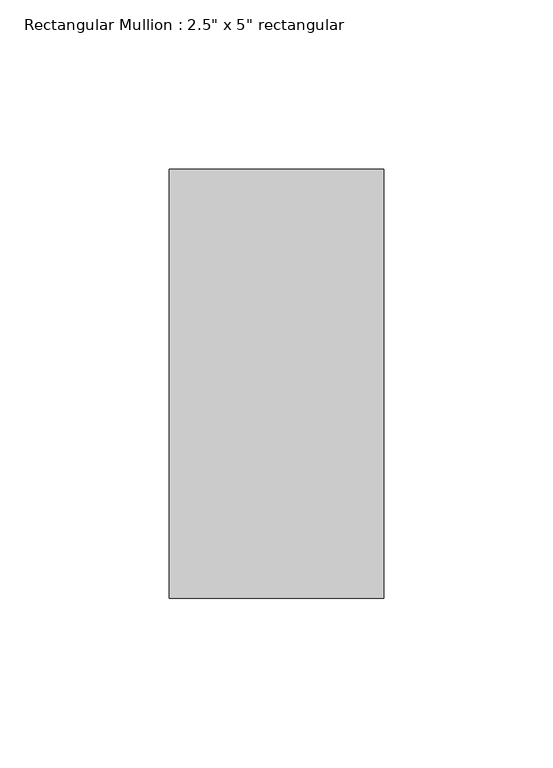
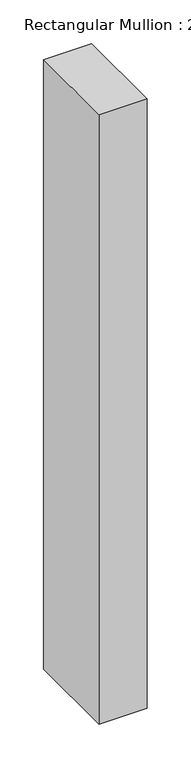
"""IFC4 building model written with IfcOpenShell, lengths in millimetres: member geometry."""

from ifc_helpers import new_model, si_unit, frame, origin, place, context, project, spatial, polyline, outline, extrude, source, transform, mapped, element, save


def member_d2e7e466(model_context):
    return source(origin(), model_context, "Body", "SweptSolid", [
        extrude(outline(polyline([(0.0, 63.5), (0.0, -63.5), (-63.5, -63.5), (-63.5, 63.5), (0.0, 63.5)])), frame((0.0, 0.0, -850.9), z_axis=(0.0, 0.0, 1.0), x_axis=(1.0, 0.0, 0.0)), (0.0, 0.0, 1.0), 850.9),
    ])


if __name__ == "__main__":
    model = new_model("IFC4")
    model_context = context("Model", 3, world=origin())
    ifc_project = project(units=[si_unit("LENGTHUNIT", "METRE", prefix="MILLI")], contexts=[model_context])
    site = spatial("IfcSite", under=ifc_project)
    building = spatial("IfcBuilding", under=site)
    placement = place(None, origin())
    member_shape = member_d2e7e466(model_context)
    element("IfcMember", 1, ObjectType="Rectangular Mullion : 2.5\" x 5\" rectangular", at=placement, inside=building, context=model_context, shape_type="MappedRepresentation", body=[
        mapped(member_shape, transform((0.0, 0.0, 0.0), x_axis=(1.0, 0.0, 0.0), y_axis=(0.0, 1.0, 0.0), z_axis=(0.0, 0.0, 1.0))),
    ])
    save(model, "model.ifc")

# Revit data of these elements
# Type "Rectangular Mullion : 2.5\" x 5\" rectangular"
#   built-in parameter 1007304 = 0.416667 (stored number, unit not read)
#   built-in parameter 1007301 = 0.104167 (stored number, unit not read)
#   built-in parameter 1007300 = 0.104167 (stored number, unit not read)
# Element 1 (IfcMember, "Rectangular Mullion : 2.5\" x 5\" rectangular")
#   Materials on its faces: "Iron, Ductile"
# Materials
#   "Iron, Ductile": class "Metal", colour RGB 0 0 0, transparency 0, Description = "Ductile cast iron", Cost = 0
